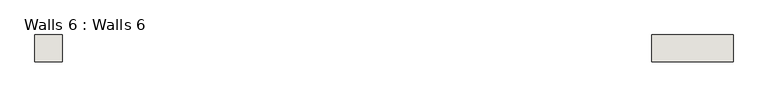
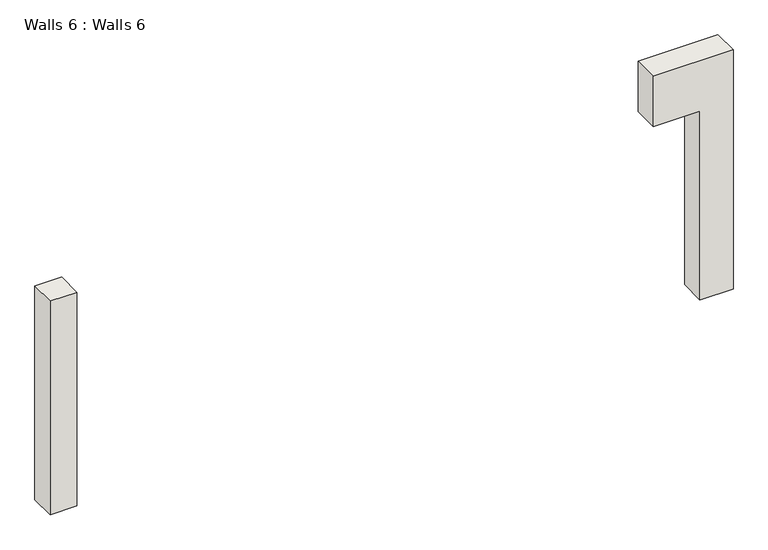
"""IFC4 building model written with IfcOpenShell, lengths in millimetres: wall geometry, Walls 6 : Walls 6."""

from ifc_helpers import new_model, si_unit, frame, origin, place, context, project, spatial, polyline, outline, extrude, source, transform, mapped, element, save


def walls_6_walls_6_895ef20a(model_context):
    return source(origin(), model_context, "Body", "SweptSolid", [
        extrude(outline(polyline([(2133.6, 515.977479), (2743.2, 515.977479), (2743.2, -398.422521), (2133.6, -398.422521), (2133.6, 134.977479), (-152.4, 134.977479), (-152.4, 515.977479), (2133.6, 515.977479)])), frame((0.0, -17634.7597971, 0.0), z_axis=(0.0, 1.0, 0.0), x_axis=(0.0, 0.0, 1.0)), (0.0, 0.0, 1.0), 301.3183587),
        extrude(outline(polyline([(-7004.022521, -17634.7597971), (-7308.822521, -17634.7597971), (-7308.822521, -17333.4414384), (-7004.022521, -17333.4414384), (-7004.022521, -17634.7597971)])), frame((0.0, 0.0, -152.4), z_axis=(0.0, 0.0, 1.0), x_axis=(1.0, 0.0, 0.0)), (0.0, 0.0, 1.0), 2590.8),
    ])


if __name__ == "__main__":
    model = new_model("IFC4")
    model_context = context("Model", 3, world=origin())
    ifc_project = project(units=[si_unit("LENGTHUNIT", "METRE", prefix="MILLI")], contexts=[model_context])
    site = spatial("IfcSite", under=ifc_project)
    building = spatial("IfcBuilding", under=site)
    placement = place(None, origin())
    walls_6_walls_6_shape = walls_6_walls_6_895ef20a(model_context)
    element("IfcWall", 1, ObjectType="Walls 6 : Walls 6", at=placement, inside=building, context=model_context, shape_type="MappedRepresentation", body=[
        mapped(walls_6_walls_6_shape, transform((0.0, 0.0, 0.0), x_axis=(1.0, 0.0, 0.0), y_axis=(0.0, 1.0, 0.0), z_axis=(0.0, 0.0, 1.0))),
    ])
    save(model, "model.ifc")

# Revit data of these elements
# Element 1 (IfcWall, "Walls 6 : Walls 6")
#   Materials on its faces: "Door - Handle", "Default Wall"
# Materials
#   "Door - Handle": colour RGB 0 0 0, transparency 0
#   "Default Wall": colour RGB 128 128 128, transparency 0
